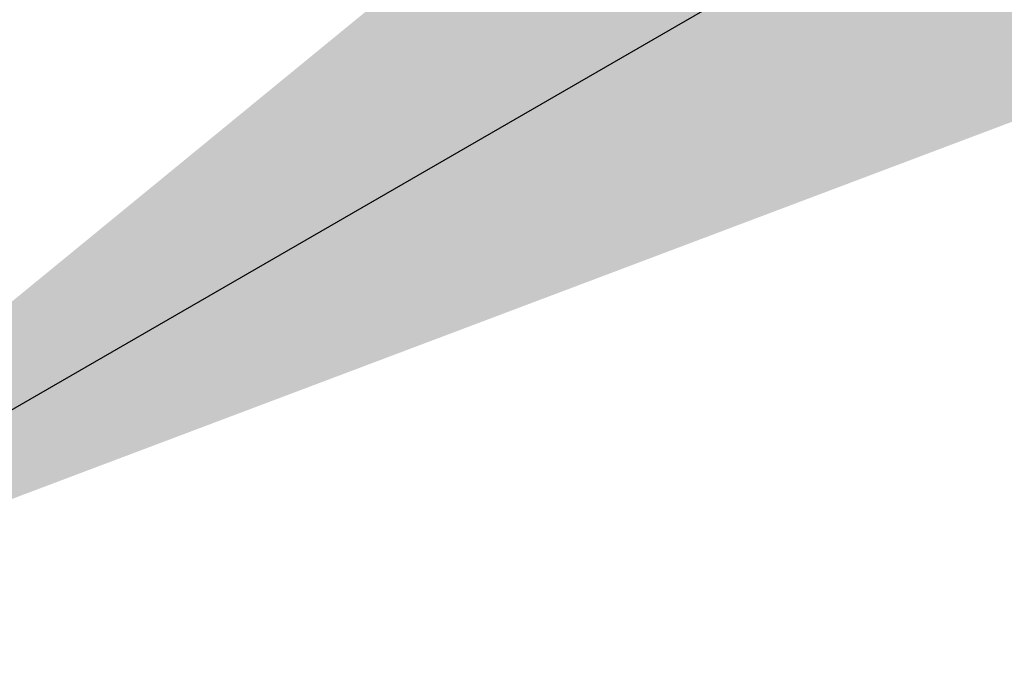
# Model space of a CAD drawing. Units: inches. Extents: x -9413 to 9703, y -9719 to 9096.
# Tile 1 of 1: x 307 to 493.3, y 154.3 to 276.8. Entities that reach past the tile are written whole.
import ezdxf
from ezdxf import colors
from ezdxf.entities.mleader import LeaderData, LeaderLine
from ezdxf.math import Vec2, Vec3

# ---------------------------------------------------------------- set-up
doc = ezdxf.new("R2010")
doc.units = ezdxf.units.IN
doc.header["$MEASUREMENT"] = 0
doc.layers.add('M-ANNO-TEXT', color=7, linetype='Continuous', lineweight=18)
doc.styles.get("Standard").update_dxf_attribs({"font": 'arial.ttf'})

msp = doc.modelspace()

# ---------------------------------------------------------------- leaders
at = {"layer": 'M-ANNO-TEXT'}
ml = msp.add_multileader_mtext('Standard', dxfattribs=at)
ml.set_content('Reheater', color=256)
ml.set_leader_properties()
ml.build(insert=Vec2(0, 0))
ml.multileader.update_dxf_attribs({"dogleg_length": 0.36, "arrow_head_size": 10000, "scale": 10})
ctx = ml.context
ctx.base_point, ctx.scale, ctx.char_height, ctx.arrow_head_size, ctx.landing_gap_size, ctx.plane_origin = Vec3(234.1414050860131, 159.7303554673012), 10, 5.4, 10000, 0.9, Vec3(221.1444910066821, 154.3050445940477)
notes = []
notes.append((ctx, [(0, (1, 1, 0), (230.5414050860131, 159.7303554673012), (1, 0), 3.599999999999999, [(0, [(221.1444910066821, 154.3050445940477)], 0, [])])]))
ctx.mtext.insert, ctx.mtext.flow_direction = Vec3(235.0414050860131, 162.4745573772603), 5
for ctx, leaders in notes:
    for number, flags, end, landing, length, lines in leaders:
        leader = LeaderData()
        leader.index, (leader.has_last_leader_line, leader.has_dogleg_vector, leader.attachment_direction) = number, flags
        leader.last_leader_point, leader.dogleg_vector, leader.dogleg_length = Vec3(end), Vec3(landing), length
        for number, points, colour, breaks in lines:
            line = LeaderLine()
            line.index, line.vertices, line.color, line.breaks = number, Vec3.list(points), colors.encode_raw_color(colour), breaks
            leader.lines.append(line)
        ctx.leaders.append(leader)

doc.saveas('drawing.dxf')
